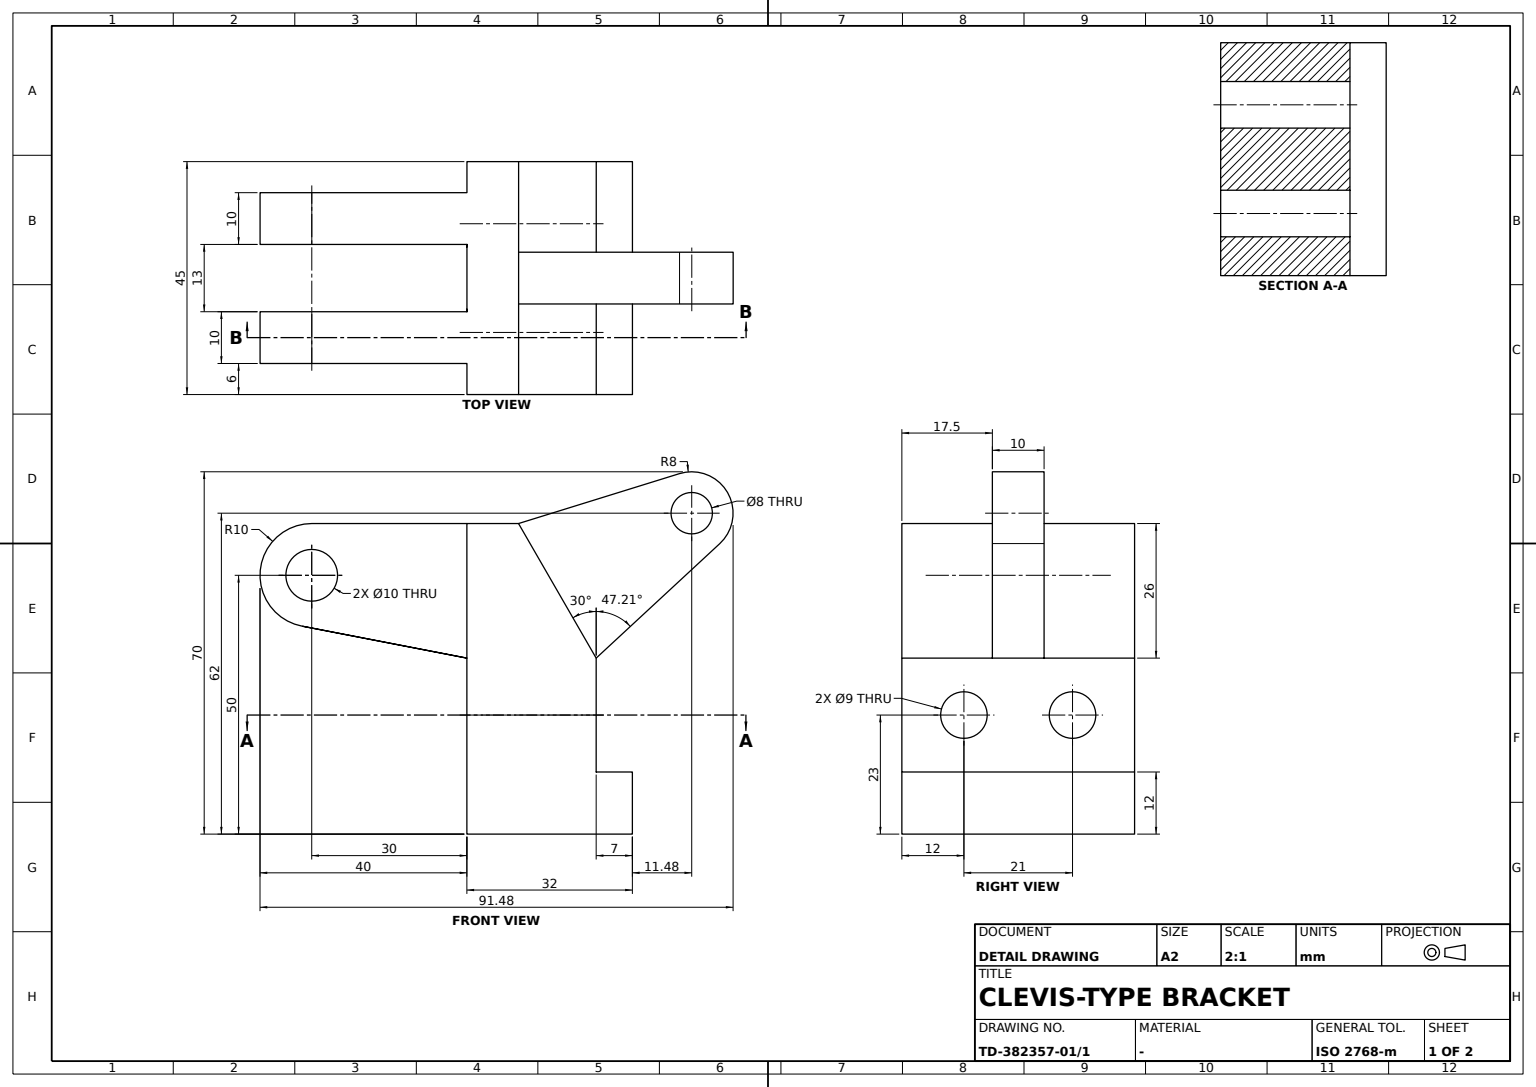
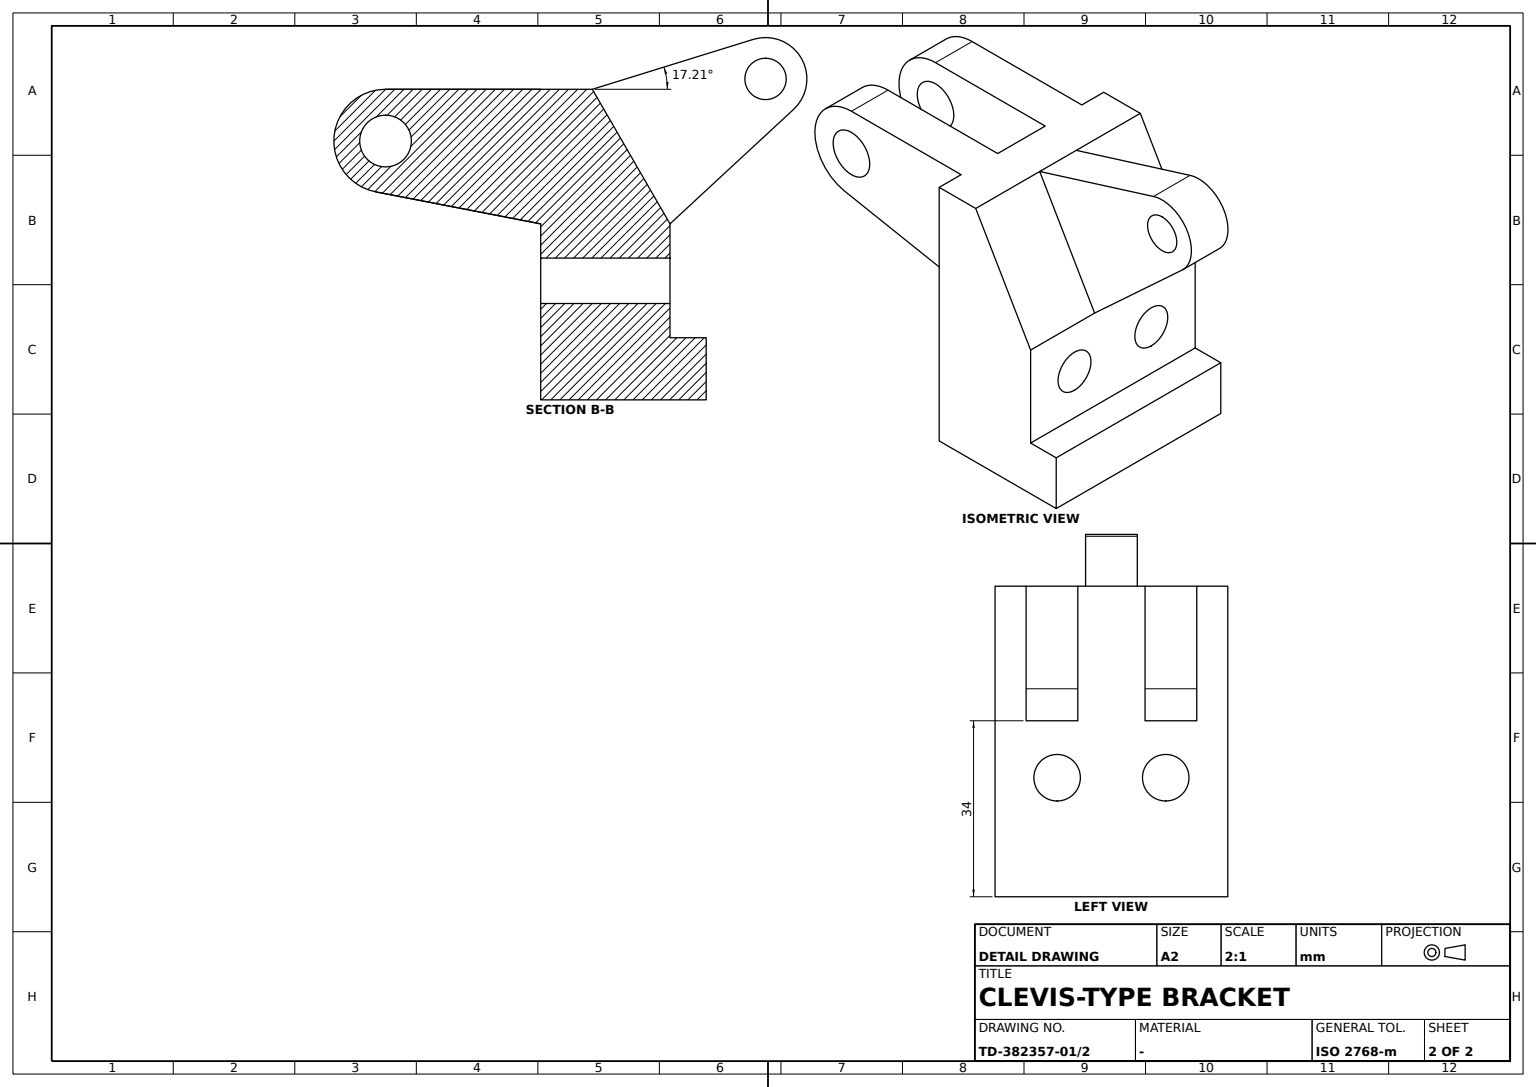
CATIA V5 part; units mm, degrees
sketch "Sketch1" plane through (0, 0, 0) normal (0, 1, 0) x (-1, 0, 0)
  line L0 (0, 0) -> (0, 12)
  line L1 (0, 12) -> (7, 12)
  line L2 (7, 12) -> (7, 34)
  line L3 (7, 34) -> (22.0111, 60)
  line L4 (22.0111, 60) -> (32, 60)
  line L5 (32, 60) -> (32, 0)
  point P0 (32, 0)
  line L6 (32, 0) -> (0, 0)
  dimension "length L0" = 12
  dimension "angle L2 L3" = 30
  dimension "length L2" = 22
  dimension "length L5" = 60
  dimension "length L6" = 32
  dimension "length L1" = 7
  constraint vertical L0 y-axis
  constraint vertical L2 y-axis
  constraint vertical L5 y-axis
  constraint horizontal L1 x-axis
  constraint horizontal L4 x-axis
  constraint horizontal L6 x-axis
  constraint coincidence P0 x-axis
extrude "Pad1" add sketch "Sketch1" along normal mid plane 45
sketch "Sketch2" plane through (0, 0, 0) normal (0, 1, 0) x (-1, 0, 0)
  line L0 (-11.4752, 62.0001) -> (14.5056, 47.0001) construction
  point P0 (14.5056, 47.0001)
  line L1 (22.0111, 60) -> (7, 34) construction
  circle A0 centre (-11.4752, 62.0001) radius 4
  arc A1 (-9.1075, 69.6417) -> (-16.9092, 56.1289) centre (-11.4752, 62.0001) ccw
  point P1 (22.0111, 60)
  line L2 (-9.1075, 69.6417) -> (22.0111, 60)
  point P2 (22.0111, 60)
  line L3 (22.0111, 60) -> (7, 34)
  point P3 (7, 34)
  line L4 (7, 34) -> (-16.9092, 56.1289)
  point P4 (7, 34)
  point P5 (22.0111, 60)
  dimension "length L0" = 30
  dimension "radius A1" = 8
  dimension "radius A0" = 4
  dimension "distance L0 P1" = 15.011
  dimension "angle L0 L3" = 90
  constraint coincidence P0 L1
  constraint coincidence P3 P4
  constraint coincidence P2 P5
  constraint tangency L2 A1
  constraint tangency L4 A1
extrude "Pad2" add sketch "Sketch2" along normal mid plane 10
sketch "Sketch3" plane through (0, 0, 0) normal (0, 1, 0) x (-1, 0, 0)
  line L0 (32, 60) -> (62, 60)
  point P0 (32, 60)
  line L1 (32, 34) -> (63.9026, 40.1827)
  point P1 (32, 34)
  point P2 (32, 60)
  line L2 (32, 0) -> (32, 60) construction
  line L3 (62, 60) -> (62, 50) construction
  arc A0 (63.9026, 40.1827) -> (62, 60) centre (62, 50) ccw
  circle A1 centre (62, 50) radius 5
  line L4 (32, 60) -> (32, 34)
  dimension "length L0" = 30
  dimension "distance P1 L0" = 26
  dimension "length L3" = 10
  dimension "radius A1" = 5
  constraint horizontal L0 x-axis
  constraint coincidence P0 P2
  constraint coincidence P1 L2
  constraint vertical L3 y-axis
  constraint vertical L4 y-axis
  constraint tangency A0 L0
  constraint tangency A0 L1
extrude "Pad3" add sketch "Sketch3" along normal mid plane 33
sketch "Sketch4" plane through (0, 0, 0) normal (0, 1, 0) x (-1, 0, 0)
  line L0 (32, 64.9698) -> (80.4459, 64.9698)
  line L1 (80.4459, 64.9698) -> (80.4459, 29.5519)
  line L2 (80.4459, 29.5519) -> (32, 29.5519)
  line L3 (32, 29.5519) -> (32, 64.9698)
  line L4 (32, 0) -> (32, 60) construction
  constraint horizontal L0 x-axis
  constraint horizontal L2 x-axis
  constraint vertical L1 y-axis
  constraint vertical L3 y-axis
  constraint coincidence L3 L4
extrude "Pocket1" cut sketch "Sketch4" along normal mid plane 13
sketch "Sketch5" plane through (0, 0, 0) normal (1, 0, 0) x (0, 1, 0)
  line L0 (-10.5, 23) -> (10.5, 23) construction
  point P0 (-10.5, 23)
  point P1 (10.5, 23)
  circle A0 centre (-10.5, 23) radius 4.5
  circle A1 centre (10.5, 23) radius 4.5
  line L1 (-22.5, 12) -> (22.5, 12) construction
  dimension "length L0" = 21
  dimension "radius A1" = 4.5
  dimension "radius A0" = 4.5
  dimension "distance L0 L1" = 11
  constraint horizontal L0 x-axis
  constraint symmetry P0 P1 y-axis
extrude "Pocket2" cut sketch "Sketch5" against normal blind 40
properties part number "11"
